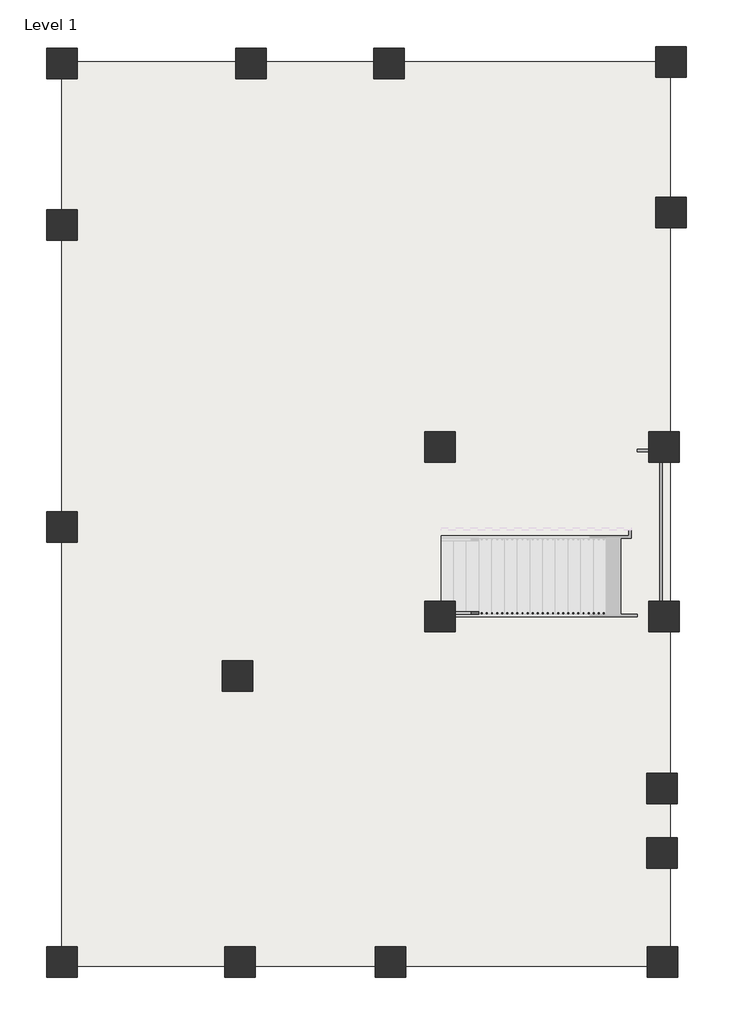
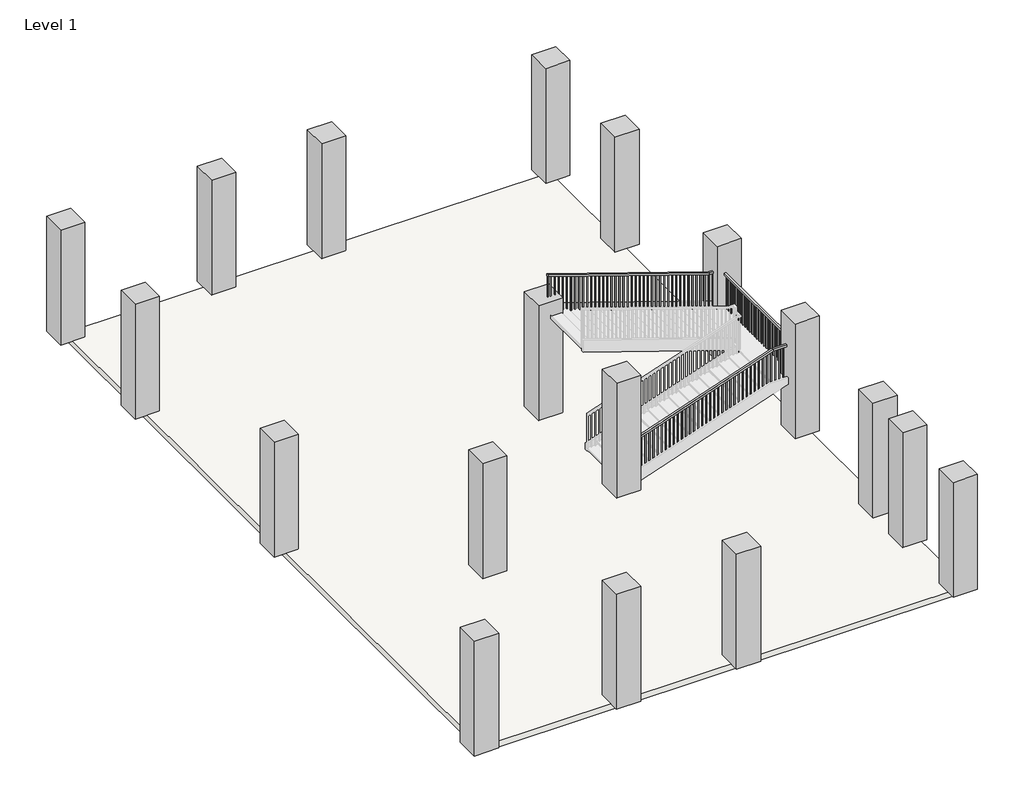
# One storey, part 1 of 2: 18 columns, 1 railing, 1 slab.
"""IFC4 building model written with IfcOpenShell, lengths in millimetres."""

from ifc_helpers import new_model, si_unit, frame, origin, origin_with_axes, place, context, project, spatial, polyline, outline, extrude, faceted_brep, element, save

model = new_model("IFC4")

# Units and contexts
model_context = context("Model", 3, world=origin())
ifc_project = project(units=[si_unit("LENGTHUNIT", "METRE", prefix="MILLI")], contexts=[model_context])

# Site, building, storey
site = spatial("IfcSite", under=ifc_project)
building = spatial("IfcBuilding", under=site)
storey = spatial("IfcBuildingStorey", under=building, Name="Level 1", Elevation=0.0)

# Columns
placement = place(None, origin())
element("IfcColumn", 1, ObjectType="Rectangular Column : 9\"x12\"/12\"x12\"", at=placement, inside=storey, context=model_context, shape_type="SweptSolid", body=[
    extrude(outline(polyline([(-5829.2560205, 9252.6670151), (-5829.2560205, 8643.0670151), (-6438.8560205, 8643.0670151), (-6438.8560205, 9252.6670151), (-5829.2560205, 9252.6670151)])), origin_with_axes(), (0.0, 0.0, 1.0), 3048.0),
])
element("IfcColumn", 2, ObjectType="Rectangular Column : 9\"x12\"/12\"x12\"", at=placement, inside=storey, context=model_context, shape_type="SweptSolid", body=[
    extrude(outline(polyline([(6350.6915654, 9284.2113669), (6350.6915654, 8674.6113669), (5741.0915654, 8674.6113669), (5741.0915654, 9284.2113669), (6350.6915654, 9284.2113669)])), origin_with_axes(), (0.0, 0.0, 1.0), 3048.0),
])
element("IfcColumn", 3, ObjectType="Rectangular Column : 9\"x12\"/12\"x12\"", at=placement, inside=storey, context=model_context, shape_type="SweptSolid", body=[
    extrude(outline(polyline([(-2044.6166288, 9252.6670151), (-2044.6166288, 8643.0670151), (-2654.2166288, 8643.0670151), (-2654.2166288, 9252.6670151), (-2044.6166288, 9252.6670151)])), origin_with_axes(), (0.0, 0.0, 1.0), 3048.0),
])
element("IfcColumn", 4, ObjectType="Rectangular Column : 9\"x12\"/12\"x12\"", at=placement, inside=storey, context=model_context, shape_type="SweptSolid", body=[
    extrude(outline(polyline([(713.9012016, 9252.6670151), (713.9012016, 8643.0670151), (104.3012016, 8643.0670151), (104.3012016, 9252.6670151), (713.9012016, 9252.6670151)])), origin_with_axes(), (0.0, 0.0, 1.0), 3048.0),
])
element("IfcColumn", 5, ObjectType="Rectangular Column : 9\"x12\"/12\"x12\"", at=placement, inside=storey, context=model_context, shape_type="SweptSolid", body=[
    extrude(outline(polyline([(-5829.2560205, 6018.6061457), (-5829.2560205, 5409.0061457), (-6438.8560205, 5409.0061457), (-6438.8560205, 6018.6061457), (-5829.2560205, 6018.6061457)])), origin_with_axes(), (0.0, 0.0, 1.0), 3048.0),
])
element("IfcColumn", 6, ObjectType="Rectangular Column : 9\"x12\"/12\"x12\"", at=placement, inside=storey, context=model_context, shape_type="SweptSolid", body=[
    extrude(outline(polyline([(-5829.1978401, -18.1127424), (-5829.1978401, -627.7127424), (-6438.7978401, -627.7127424), (-6438.7978401, -18.1127424), (-5829.1978401, -18.1127424)])), origin_with_axes(), (0.0, 0.0, 1.0), 3048.0),
])
element("IfcColumn", 7, ObjectType="Rectangular Column : 9\"x12\"/12\"x12\"", at=placement, inside=storey, context=model_context, shape_type="SweptSolid", body=[
    extrude(outline(polyline([(-5826.9839448, -8713.9734342), (-5826.9839448, -9323.5734342), (-6436.5839448, -9323.5734342), (-6436.5839448, -8713.9734342), (-5826.9839448, -8713.9734342)])), origin_with_axes(), (0.0, 0.0, 1.0), 3048.0),
])
element("IfcColumn", 8, ObjectType="Rectangular Column : 9\"x12\"/12\"x12\"", at=placement, inside=storey, context=model_context, shape_type="SweptSolid", body=[
    extrude(outline(polyline([(-2270.3220989, -8713.9734342), (-2270.3220989, -9323.5734342), (-2879.9220989, -9323.5734342), (-2879.9220989, -8713.9734342), (-2270.3220989, -8713.9734342)])), origin_with_axes(), (0.0, 0.0, 1.0), 3048.0),
])
element("IfcColumn", 9, ObjectType="Rectangular Column : 9\"x12\"/12\"x12\"", at=placement, inside=storey, context=model_context, shape_type="SweptSolid", body=[
    extrude(outline(polyline([(745.5939638, -8713.9734342), (745.5939638, -9323.5734342), (135.9939638, -9323.5734342), (135.9939638, -8713.9734342), (745.5939638, -8713.9734342)])), origin_with_axes(), (0.0, 0.0, 1.0), 3048.0),
])
element("IfcColumn", 10, ObjectType="Rectangular Column : 9\"x12\"/12\"x12\"", at=placement, inside=storey, context=model_context, shape_type="SweptSolid", body=[
    extrude(outline(polyline([(6178.8473287, -8713.9734342), (6178.8473287, -9323.5734342), (5569.2473287, -9323.5734342), (5569.2473287, -8713.9734342), (6178.8473287, -8713.9734342)])), origin_with_axes(), (0.0, 0.0, 1.0), 3048.0),
])
element("IfcColumn", 11, ObjectType="Rectangular Column : 9\"x12\"/12\"x12\"", at=placement, inside=storey, context=model_context, shape_type="SweptSolid", body=[
    extrude(outline(polyline([(6172.2396412, -6530.895318), (6172.2396412, -7140.495318), (5562.6396412, -7140.495318), (5562.6396412, -6530.895318), (6172.2396412, -6530.895318)])), origin_with_axes(), (0.0, 0.0, 1.0), 3048.0),
])
element("IfcColumn", 12, ObjectType="Rectangular Column : 9\"x12\"/12\"x12\"", at=placement, inside=storey, context=model_context, shape_type="SweptSolid", body=[
    extrude(outline(polyline([(6172.2396412, -5240.916233), (6172.2396412, -5850.516233), (5562.6396412, -5850.516233), (5562.6396412, -5240.916233), (6172.2396412, -5240.916233)])), origin_with_axes(), (0.0, 0.0, 1.0), 3048.0),
])
element("IfcColumn", 13, ObjectType="Rectangular Column : 9\"x12\"/12\"x12\"", at=placement, inside=storey, context=model_context, shape_type="SweptSolid", body=[
    extrude(outline(polyline([(6208.2949572, -1801.6977001), (6208.2949572, -2411.2977001), (5598.6949572, -2411.2977001), (5598.6949572, -1801.6977001), (6208.2949572, -1801.6977001)])), origin_with_axes(), (0.0, 0.0, 1.0), 3048.0),
])
element("IfcColumn", 14, ObjectType="Rectangular Column : 9\"x12\"/12\"x12\"", at=placement, inside=storey, context=model_context, shape_type="SweptSolid", body=[
    extrude(outline(polyline([(6208.2949572, 1586.0589984), (6208.2949572, 976.4589984), (5598.6949572, 976.4589984), (5598.6949572, 1586.0589984), (6208.2949572, 1586.0589984)])), origin_with_axes(), (0.0, 0.0, 1.0), 3048.0),
])
element("IfcColumn", 15, ObjectType="Rectangular Column : 9\"x12\"/12\"x12\"", at=placement, inside=storey, context=model_context, shape_type="SweptSolid", body=[
    extrude(outline(polyline([(6350.6915654, 6275.5882388), (6350.6915654, 5665.9882388), (5741.0915654, 5665.9882388), (5741.0915654, 6275.5882388), (6350.6915654, 6275.5882388)])), origin_with_axes(), (0.0, 0.0, 1.0), 3048.0),
])
element("IfcColumn", 16, ObjectType="Rectangular Column : 9\"x12\"/12\"x12\"", at=placement, inside=storey, context=model_context, shape_type="SweptSolid", body=[
    extrude(outline(polyline([(1728.7932247, 1586.0589984), (1728.7932247, 976.4589984), (1119.1932247, 976.4589984), (1119.1932247, 1586.0589984), (1728.7932247, 1586.0589984)])), origin_with_axes(), (0.0, 0.0, 1.0), 3048.0),
])
element("IfcColumn", 17, ObjectType="Rectangular Column : 9\"x12\"/12\"x12\"", at=placement, inside=storey, context=model_context, shape_type="SweptSolid", body=[
    extrude(outline(polyline([(1728.7932247, -1801.6977001), (1728.7932247, -2411.2977001), (1119.1932247, -2411.2977001), (1119.1932247, -1801.6977001), (1728.7932247, -1801.6977001)])), origin_with_axes(), (0.0, 0.0, 1.0), 3048.0),
])
element("IfcColumn", 18, ObjectType="Rectangular Column : 9\"x12\"/12\"x12\"", at=placement, inside=storey, context=model_context, shape_type="SweptSolid", body=[
    extrude(outline(polyline([(-2316.8197661, -2995.5861861), (-2316.8197661, -3605.1861861), (-2926.4197661, -3605.1861861), (-2926.4197661, -2995.5861861), (-2316.8197661, -2995.5861861)])), origin_with_axes(), (0.0, 0.0, 1.0), 3048.0),
])

# Railing
element("IfcRailing", 19, ObjectType="Handrail - Rectangular", at=placement, inside=storey, context=model_context, shape_type="SolidModel", body=[
    faceted_brep([(1449.3932247, -2014.4659014, 1000.125), (1449.3932247, -2014.4659014, 946.4913852), (1449.3932247, -2065.2659014, 946.4913852), (1449.3932247, -2065.2659014, 1000.125), (5246.6669505, -2014.4659014, 2286.0), (5255.0348019, -2014.4659014, 2235.2), (5255.0348019, -2065.2659014, 2235.2), (5246.6669505, -2065.2659014, 2286.0), (5771.4548051, -2014.4659014, 2286.0), (5771.4548051, -2014.4659014, 2235.2), (5822.2548051, -2065.2659014, 2235.2), (5822.2548051, -2065.2659014, 2286.0), (5771.4548051, 1135.1340986, 2286.0), (5771.4548051, 1135.1340986, 2235.2), (5822.2548051, 1185.9340986, 2235.2), (5822.2548051, 1185.9340986, 2286.0), (5499.8185322, 1135.1340986, 2286.0), (5491.4506807, 1135.1340986, 2235.2), (5491.4506807, 1185.9340986, 2235.2), (5499.8185322, 1185.9340986, 2286.0), (1449.3932247, 1135.1340986, 3657.6), (1449.3932247, 1185.9340986, 3657.6), (1449.3932247, 1185.9340986, 3603.9663852), (1449.3932247, 1135.1340986, 3603.9663852)], [[[0, 1, 2, 3]], [[1, 0, 4, 5]], [[2, 1, 5, 6]], [[3, 2, 6, 7]], [[0, 3, 7, 4]], [[5, 4, 8, 9]], [[6, 5, 9, 10]], [[7, 6, 10, 11]], [[4, 7, 11, 8]], [[9, 8, 12, 13]], [[10, 9, 13, 14]], [[11, 10, 14, 15]], [[8, 11, 15, 12]], [[13, 12, 16, 17]], [[14, 13, 17, 18]], [[15, 14, 18, 19]], [[12, 15, 19, 16]], [[20, 21, 22, 23]], [[17, 16, 20, 23]], [[18, 17, 23, 22]], [[19, 18, 22, 21]], [[16, 19, 21, 20]]]),
    extrude(outline(polyline([(3573.5618562, 1539.1798051), (3580.0127788, 1520.1298051), (2657.475, 1520.1298051), (2657.475, 1539.1798051), (3573.5618562, 1539.1798051)])), frame((0.0, 1151.0090986, 0.0), z_axis=(0.0, 1.0, 0.0), x_axis=(0.0, 0.0, 1.0)), (0.0, 0.0, 1.0), 19.05),
    extrude(outline(polyline([(3539.1569359, 1640.7798051), (3545.6078585, 1621.7298051), (2657.475, 1621.7298051), (2657.475, 1640.7798051), (3539.1569359, 1640.7798051)])), frame((0.0, 1151.0090986, 0.0), z_axis=(0.0, 1.0, 0.0), x_axis=(0.0, 0.0, 1.0)), (0.0, 0.0, 1.0), 19.05),
    extrude(outline(polyline([(3504.7520156, 1742.3798051), (3511.2029381, 1723.3298051), (2571.75, 1723.3298051), (2571.75, 1742.3798051), (3504.7520156, 1742.3798051)])), frame((0.0, 1151.0090986, 0.0), z_axis=(0.0, 1.0, 0.0), x_axis=(0.0, 0.0, 1.0)), (0.0, 0.0, 1.0), 19.05),
    extrude(outline(polyline([(3470.3470953, 1843.9798051), (3476.7980178, 1824.9298051), (2571.75, 1824.9298051), (2571.75, 1843.9798051), (3470.3470953, 1843.9798051)])), frame((0.0, 1151.0090986, 0.0), z_axis=(0.0, 1.0, 0.0), x_axis=(0.0, 0.0, 1.0)), (0.0, 0.0, 1.0), 19.05),
    extrude(outline(polyline([(3435.9421749, 1945.5798051), (3442.3930975, 1926.5298051), (2571.75, 1926.5298051), (2571.75, 1945.5798051), (3435.9421749, 1945.5798051)])), frame((0.0, 1151.0090986, 0.0), z_axis=(0.0, 1.0, 0.0), x_axis=(0.0, 0.0, 1.0)), (0.0, 0.0, 1.0), 19.05),
    extrude(outline(polyline([(3401.5372546, 2047.1798051), (3407.9881772, 2028.1298051), (2486.025, 2028.1298051), (2486.025, 2047.1798051), (3401.5372546, 2047.1798051)])), frame((0.0, 1151.0090986, 0.0), z_axis=(0.0, 1.0, 0.0), x_axis=(0.0, 0.0, 1.0)), (0.0, 0.0, 1.0), 19.05),
    extrude(outline(polyline([(3367.1323343, 2148.7798051), (3373.5832568, 2129.7298051), (2486.025, 2129.7298051), (2486.025, 2148.7798051), (3367.1323343, 2148.7798051)])), frame((0.0, 1151.0090986, 0.0), z_axis=(0.0, 1.0, 0.0), x_axis=(0.0, 0.0, 1.0)), (0.0, 0.0, 1.0), 19.05),
    extrude(outline(polyline([(3332.7274139, 2250.3798051), (3339.1783365, 2231.3298051), (2400.3, 2231.3298051), (2400.3, 2250.3798051), (3332.7274139, 2250.3798051)])), frame((0.0, 1151.0090986, 0.0), z_axis=(0.0, 1.0, 0.0), x_axis=(0.0, 0.0, 1.0)), (0.0, 0.0, 1.0), 19.05),
    extrude(outline(polyline([(3298.3224936, 2351.9798051), (3304.7734162, 2332.9298051), (2400.3, 2332.9298051), (2400.3, 2351.9798051), (3298.3224936, 2351.9798051)])), frame((0.0, 1151.0090986, 0.0), z_axis=(0.0, 1.0, 0.0), x_axis=(0.0, 0.0, 1.0)), (0.0, 0.0, 1.0), 19.05),
    extrude(outline(polyline([(3263.9175733, 2453.5798051), (3270.3684958, 2434.5298051), (2400.3, 2434.5298051), (2400.3, 2453.5798051), (3263.9175733, 2453.5798051)])), frame((0.0, 1151.0090986, 0.0), z_axis=(0.0, 1.0, 0.0), x_axis=(0.0, 0.0, 1.0)), (0.0, 0.0, 1.0), 19.05),
    extrude(outline(polyline([(3229.512653, 2555.1798051), (3235.9635755, 2536.1298051), (2314.575, 2536.1298051), (2314.575, 2555.1798051), (3229.512653, 2555.1798051)])), frame((0.0, 1151.0090986, 0.0), z_axis=(0.0, 1.0, 0.0), x_axis=(0.0, 0.0, 1.0)), (0.0, 0.0, 1.0), 19.05),
    extrude(outline(polyline([(3195.1077326, 2656.7798051), (3201.5586552, 2637.7298051), (2314.575, 2637.7298051), (2314.575, 2656.7798051), (3195.1077326, 2656.7798051)])), frame((0.0, 1151.0090986, 0.0), z_axis=(0.0, 1.0, 0.0), x_axis=(0.0, 0.0, 1.0)), (0.0, 0.0, 1.0), 19.05),
    extrude(outline(polyline([(3160.7028123, 2758.3798051), (3167.1537349, 2739.3298051), (2228.85, 2739.3298051), (2228.85, 2758.3798051), (3160.7028123, 2758.3798051)])), frame((0.0, 1151.0090986, 0.0), z_axis=(0.0, 1.0, 0.0), x_axis=(0.0, 0.0, 1.0)), (0.0, 0.0, 1.0), 19.05),
    extrude(outline(polyline([(3126.297892, 2859.9798051), (3132.7488145, 2840.9298051), (2228.85, 2840.9298051), (2228.85, 2859.9798051), (3126.297892, 2859.9798051)])), frame((0.0, 1151.0090986, 0.0), z_axis=(0.0, 1.0, 0.0), x_axis=(0.0, 0.0, 1.0)), (0.0, 0.0, 1.0), 19.05),
    extrude(outline(polyline([(3091.8929716, 2961.5798051), (3098.3438942, 2942.5298051), (2228.85, 2942.5298051), (2228.85, 2961.5798051), (3091.8929716, 2961.5798051)])), frame((0.0, 1151.0090986, 0.0), z_axis=(0.0, 1.0, 0.0), x_axis=(0.0, 0.0, 1.0)), (0.0, 0.0, 1.0), 19.05),
    extrude(outline(polyline([(3057.4880513, 3063.1798051), (3063.9389739, 3044.1298051), (2143.125, 3044.1298051), (2143.125, 3063.1798051), (3057.4880513, 3063.1798051)])), frame((0.0, 1151.0090986, 0.0), z_axis=(0.0, 1.0, 0.0), x_axis=(0.0, 0.0, 1.0)), (0.0, 0.0, 1.0), 19.05),
    extrude(outline(polyline([(3023.083131, 3164.7798051), (3029.5340535, 3145.7298051), (2143.125, 3145.7298051), (2143.125, 3164.7798051), (3023.083131, 3164.7798051)])), frame((0.0, 1151.0090986, 0.0), z_axis=(0.0, 1.0, 0.0), x_axis=(0.0, 0.0, 1.0)), (0.0, 0.0, 1.0), 19.05),
    extrude(outline(polyline([(2988.6782106, 3266.3798051), (2995.1291332, 3247.3298051), (2057.4, 3247.3298051), (2057.4, 3266.3798051), (2988.6782106, 3266.3798051)])), frame((0.0, 1151.0090986, 0.0), z_axis=(0.0, 1.0, 0.0), x_axis=(0.0, 0.0, 1.0)), (0.0, 0.0, 1.0), 19.05),
    extrude(outline(polyline([(2954.2732903, 3367.9798051), (2960.7242129, 3348.9298051), (2057.4, 3348.9298051), (2057.4, 3367.9798051), (2954.2732903, 3367.9798051)])), frame((0.0, 1151.0090986, 0.0), z_axis=(0.0, 1.0, 0.0), x_axis=(0.0, 0.0, 1.0)), (0.0, 0.0, 1.0), 19.05),
    extrude(outline(polyline([(2919.86837, 3469.5798051), (2926.3192926, 3450.5298051), (2057.4, 3450.5298051), (2057.4, 3469.5798051), (2919.86837, 3469.5798051)])), frame((0.0, 1151.0090986, 0.0), z_axis=(0.0, 1.0, 0.0), x_axis=(0.0, 0.0, 1.0)), (0.0, 0.0, 1.0), 19.05),
    extrude(outline(polyline([(2885.4634497, 3571.1798051), (2891.9143722, 3552.1298051), (1971.675, 3552.1298051), (1971.675, 3571.1798051), (2885.4634497, 3571.1798051)])), frame((0.0, 1151.0090986, 0.0), z_axis=(0.0, 1.0, 0.0), x_axis=(0.0, 0.0, 1.0)), (0.0, 0.0, 1.0), 19.05),
    extrude(outline(polyline([(2851.0585293, 3672.7798051), (2857.5094519, 3653.7298051), (1971.675, 3653.7298051), (1971.675, 3672.7798051), (2851.0585293, 3672.7798051)])), frame((0.0, 1151.0090986, 0.0), z_axis=(0.0, 1.0, 0.0), x_axis=(0.0, 0.0, 1.0)), (0.0, 0.0, 1.0), 19.05),
    extrude(outline(polyline([(2816.653609, 3774.3798051), (2823.1045316, 3755.3298051), (1885.95, 3755.3298051), (1885.95, 3774.3798051), (2816.653609, 3774.3798051)])), frame((0.0, 1151.0090986, 0.0), z_axis=(0.0, 1.0, 0.0), x_axis=(0.0, 0.0, 1.0)), (0.0, 0.0, 1.0), 19.05),
    extrude(outline(polyline([(2782.2486887, 3875.9798051), (2788.6996112, 3856.9298051), (1885.95, 3856.9298051), (1885.95, 3875.9798051), (2782.2486887, 3875.9798051)])), frame((0.0, 1151.0090986, 0.0), z_axis=(0.0, 1.0, 0.0), x_axis=(0.0, 0.0, 1.0)), (0.0, 0.0, 1.0), 19.05),
    extrude(outline(polyline([(2747.8437683, 3977.5798051), (2754.2946909, 3958.5298051), (1885.95, 3958.5298051), (1885.95, 3977.5798051), (2747.8437683, 3977.5798051)])), frame((0.0, 1151.0090986, 0.0), z_axis=(0.0, 1.0, 0.0), x_axis=(0.0, 0.0, 1.0)), (0.0, 0.0, 1.0), 19.05),
    extrude(outline(polyline([(2713.438848, 4079.1798051), (2719.8897706, 4060.1298051), (1800.225, 4060.1298051), (1800.225, 4079.1798051), (2713.438848, 4079.1798051)])), frame((0.0, 1151.0090986, 0.0), z_axis=(0.0, 1.0, 0.0), x_axis=(0.0, 0.0, 1.0)), (0.0, 0.0, 1.0), 19.05),
    extrude(outline(polyline([(2679.0339277, 4180.7798051), (2685.4848503, 4161.7298051), (1800.225, 4161.7298051), (1800.225, 4180.7798051), (2679.0339277, 4180.7798051)])), frame((0.0, 1151.0090986, 0.0), z_axis=(0.0, 1.0, 0.0), x_axis=(0.0, 0.0, 1.0)), (0.0, 0.0, 1.0), 19.05),
    extrude(outline(polyline([(2644.6290074, 4282.3798051), (2651.0799299, 4263.3298051), (1714.5, 4263.3298051), (1714.5, 4282.3798051), (2644.6290074, 4282.3798051)])), frame((0.0, 1151.0090986, 0.0), z_axis=(0.0, 1.0, 0.0), x_axis=(0.0, 0.0, 1.0)), (0.0, 0.0, 1.0), 19.05),
    extrude(outline(polyline([(2610.224087, 4383.9798051), (2616.6750096, 4364.9298051), (1714.5, 4364.9298051), (1714.5, 4383.9798051), (2610.224087, 4383.9798051)])), frame((0.0, 1151.0090986, 0.0), z_axis=(0.0, 1.0, 0.0), x_axis=(0.0, 0.0, 1.0)), (0.0, 0.0, 1.0), 19.05),
    extrude(outline(polyline([(2575.8191667, 4485.5798051), (2582.2700893, 4466.5298051), (1714.5, 4466.5298051), (1714.5, 4485.5798051), (2575.8191667, 4485.5798051)])), frame((0.0, 1151.0090986, 0.0), z_axis=(0.0, 1.0, 0.0), x_axis=(0.0, 0.0, 1.0)), (0.0, 0.0, 1.0), 19.05),
    extrude(outline(polyline([(2541.4142464, 4587.1798051), (2547.8651689, 4568.1298051), (1628.775, 4568.1298051), (1628.775, 4587.1798051), (2541.4142464, 4587.1798051)])), frame((0.0, 1151.0090986, 0.0), z_axis=(0.0, 1.0, 0.0), x_axis=(0.0, 0.0, 1.0)), (0.0, 0.0, 1.0), 19.05),
    extrude(outline(polyline([(2507.009326, 4688.7798051), (2513.4602486, 4669.7298051), (1628.775, 4669.7298051), (1628.775, 4688.7798051), (2507.009326, 4688.7798051)])), frame((0.0, 1151.0090986, 0.0), z_axis=(0.0, 1.0, 0.0), x_axis=(0.0, 0.0, 1.0)), (0.0, 0.0, 1.0), 19.05),
    extrude(outline(polyline([(2472.6044057, 4790.3798051), (2479.0553283, 4771.3298051), (1543.05, 4771.3298051), (1543.05, 4790.3798051), (2472.6044057, 4790.3798051)])), frame((0.0, 1151.0090986, 0.0), z_axis=(0.0, 1.0, 0.0), x_axis=(0.0, 0.0, 1.0)), (0.0, 0.0, 1.0), 19.05),
    extrude(outline(polyline([(2438.1994854, 4891.9798051), (2444.6504079, 4872.9298051), (1543.05, 4872.9298051), (1543.05, 4891.9798051), (2438.1994854, 4891.9798051)])), frame((0.0, 1151.0090986, 0.0), z_axis=(0.0, 1.0, 0.0), x_axis=(0.0, 0.0, 1.0)), (0.0, 0.0, 1.0), 19.05),
    extrude(outline(polyline([(2403.8163852, 4993.5798051), (2410.2673078, 4974.5298051), (1543.05, 4974.5298051), (1543.05, 4993.5798051), (2403.8163852, 4993.5798051)])), frame((0.0, 1151.0090986, 0.0), z_axis=(0.0, 1.0, 0.0), x_axis=(0.0, 0.0, 1.0)), (0.0, 0.0, 1.0), 19.05),
    extrude(outline(polyline([(2369.3896447, 5095.1798051), (2375.8405673, 5076.1298051), (1457.325, 5076.1298051), (1457.325, 5095.1798051), (2369.3896447, 5095.1798051)])), frame((0.0, 1151.0090986, 0.0), z_axis=(0.0, 1.0, 0.0), x_axis=(0.0, 0.0, 1.0)), (0.0, 0.0, 1.0), 19.05),
    extrude(outline(polyline([(2334.9847244, 5196.7798051), (2341.435647, 5177.7298051), (1457.325, 5177.7298051), (1457.325, 5196.7798051), (2334.9847244, 5196.7798051)])), frame((0.0, 1151.0090986, 0.0), z_axis=(0.0, 1.0, 0.0), x_axis=(0.0, 0.0, 1.0)), (0.0, 0.0, 1.0), 19.05),
    extrude(outline(polyline([(2300.5798041, 5298.3798051), (2307.0307266, 5279.3298051), (1371.6, 5279.3298051), (1371.6, 5298.3798051), (2300.5798041, 5298.3798051)])), frame((0.0, 1151.0090986, 0.0), z_axis=(0.0, 1.0, 0.0), x_axis=(0.0, 0.0, 1.0)), (0.0, 0.0, 1.0), 19.05),
    extrude(outline(polyline([(2266.1748837, 5399.9798051), (2272.6258063, 5380.9298051), (1371.6, 5380.9298051), (1371.6, 5399.9798051), (2266.1748837, 5399.9798051)])), frame((0.0, 1151.0090986, 0.0), z_axis=(0.0, 1.0, 0.0), x_axis=(0.0, 0.0, 1.0)), (0.0, 0.0, 1.0), 19.05),
    extrude(outline(polyline([(2231.7699634, 5501.5798051), (2238.220886, 5482.5298051), (1371.6, 5482.5298051), (1371.6, 5501.5798051), (2231.7699634, 5501.5798051)])), frame((0.0, 1151.0090986, 0.0), z_axis=(0.0, 1.0, 0.0), x_axis=(0.0, 0.0, 1.0)), (0.0, 0.0, 1.0), 19.05),
    extrude(outline(polyline([(5603.1798051, 1170.0590986), (5603.1798051, 1151.0090986), (5584.1298051, 1151.0090986), (5584.1298051, 1170.0590986), (5603.1798051, 1170.0590986)])), frame((0.0, 0.0, 1371.6), z_axis=(0.0, 0.0, 1.0), x_axis=(1.0, 0.0, 0.0)), (0.0, 0.0, 1.0), 863.6),
    extrude(outline(polyline([(5704.7798051, 1170.0590986), (5704.7798051, 1151.0090986), (5685.7298051, 1151.0090986), (5685.7298051, 1170.0590986), (5704.7798051, 1170.0590986)])), frame((0.0, 0.0, 1371.6), z_axis=(0.0, 0.0, 1.0), x_axis=(1.0, 0.0, 0.0)), (0.0, 0.0, 1.0), 863.6),
    extrude(outline(polyline([(5806.3798051, 1100.2090986), (5787.3298051, 1100.2090986), (5787.3298051, 1119.2590986), (5806.3798051, 1119.2590986), (5806.3798051, 1100.2090986)])), frame((0.0, 0.0, 1371.6), z_axis=(0.0, 0.0, 1.0), x_axis=(1.0, 0.0, 0.0)), (0.0, 0.0, 1.0), 863.6),
    extrude(outline(polyline([(5806.3798051, 998.6090986), (5787.3298051, 998.6090986), (5787.3298051, 1017.6590986), (5806.3798051, 1017.6590986), (5806.3798051, 998.6090986)])), frame((0.0, 0.0, 1371.6), z_axis=(0.0, 0.0, 1.0), x_axis=(1.0, 0.0, 0.0)), (0.0, 0.0, 1.0), 863.6),
    extrude(outline(polyline([(5806.3798051, 897.0090986), (5787.3298051, 897.0090986), (5787.3298051, 916.0590986), (5806.3798051, 916.0590986), (5806.3798051, 897.0090986)])), frame((0.0, 0.0, 1371.6), z_axis=(0.0, 0.0, 1.0), x_axis=(1.0, 0.0, 0.0)), (0.0, 0.0, 1.0), 863.6),
    extrude(outline(polyline([(5806.3798051, 795.4090986), (5787.3298051, 795.4090986), (5787.3298051, 814.4590986), (5806.3798051, 814.4590986), (5806.3798051, 795.4090986)])), frame((0.0, 0.0, 1371.6), z_axis=(0.0, 0.0, 1.0), x_axis=(1.0, 0.0, 0.0)), (0.0, 0.0, 1.0), 863.6),
    extrude(outline(polyline([(5806.3798051, 693.8090986), (5787.3298051, 693.8090986), (5787.3298051, 712.8590986), (5806.3798051, 712.8590986), (5806.3798051, 693.8090986)])), frame((0.0, 0.0, 1371.6), z_axis=(0.0, 0.0, 1.0), x_axis=(1.0, 0.0, 0.0)), (0.0, 0.0, 1.0), 863.6),
    extrude(outline(polyline([(5806.3798051, 592.2090986), (5787.3298051, 592.2090986), (5787.3298051, 611.2590986), (5806.3798051, 611.2590986), (5806.3798051, 592.2090986)])), frame((0.0, 0.0, 1371.6), z_axis=(0.0, 0.0, 1.0), x_axis=(1.0, 0.0, 0.0)), (0.0, 0.0, 1.0), 863.6),
    extrude(outline(polyline([(5806.3798051, 490.6090986), (5787.3298051, 490.6090986), (5787.3298051, 509.6590986), (5806.3798051, 509.6590986), (5806.3798051, 490.6090986)])), frame((0.0, 0.0, 1371.6), z_axis=(0.0, 0.0, 1.0), x_axis=(1.0, 0.0, 0.0)), (0.0, 0.0, 1.0), 863.6),
    extrude(outline(polyline([(5806.3798051, 389.0090986), (5787.3298051, 389.0090986), (5787.3298051, 408.0590986), (5806.3798051, 408.0590986), (5806.3798051, 389.0090986)])), frame((0.0, 0.0, 1371.6), z_axis=(0.0, 0.0, 1.0), x_axis=(1.0, 0.0, 0.0)), (0.0, 0.0, 1.0), 863.6),
    extrude(outline(polyline([(5806.3798051, 287.4090986), (5787.3298051, 287.4090986), (5787.3298051, 306.4590986), (5806.3798051, 306.4590986), (5806.3798051, 287.4090986)])), frame((0.0, 0.0, 1371.6), z_axis=(0.0, 0.0, 1.0), x_axis=(1.0, 0.0, 0.0)), (0.0, 0.0, 1.0), 863.6),
    extrude(outline(polyline([(5806.3798051, 185.8090986), (5787.3298051, 185.8090986), (5787.3298051, 204.8590986), (5806.3798051, 204.8590986), (5806.3798051, 185.8090986)])), frame((0.0, 0.0, 1371.6), z_axis=(0.0, 0.0, 1.0), x_axis=(1.0, 0.0, 0.0)), (0.0, 0.0, 1.0), 863.6),
    extrude(outline(polyline([(5806.3798051, 84.2090986), (5787.3298051, 84.2090986), (5787.3298051, 103.2590986), (5806.3798051, 103.2590986), (5806.3798051, 84.2090986)])), frame((0.0, 0.0, 1371.6), z_axis=(0.0, 0.0, 1.0), x_axis=(1.0, 0.0, 0.0)), (0.0, 0.0, 1.0), 863.6),
    extrude(outline(polyline([(5806.3798051, -17.3909014), (5787.3298051, -17.3909014), (5787.3298051, 1.6590986), (5806.3798051, 1.6590986), (5806.3798051, -17.3909014)])), frame((0.0, 0.0, 1371.6), z_axis=(0.0, 0.0, 1.0), x_axis=(1.0, 0.0, 0.0)), (0.0, 0.0, 1.0), 863.6),
    extrude(outline(polyline([(5806.3798051, -118.9909014), (5787.3298051, -118.9909014), (5787.3298051, -99.9409014), (5806.3798051, -99.9409014), (5806.3798051, -118.9909014)])), frame((0.0, 0.0, 1371.6), z_axis=(0.0, 0.0, 1.0), x_axis=(1.0, 0.0, 0.0)), (0.0, 0.0, 1.0), 863.6),
    extrude(outline(polyline([(5806.3798051, -220.5909014), (5787.3298051, -220.5909014), (5787.3298051, -201.5409014), (5806.3798051, -201.5409014), (5806.3798051, -220.5909014)])), frame((0.0, 0.0, 1371.6), z_axis=(0.0, 0.0, 1.0), x_axis=(1.0, 0.0, 0.0)), (0.0, 0.0, 1.0), 863.6),
    extrude(outline(polyline([(5806.3798051, -322.1909014), (5787.3298051, -322.1909014), (5787.3298051, -303.1409014), (5806.3798051, -303.1409014), (5806.3798051, -322.1909014)])), frame((0.0, 0.0, 1371.6), z_axis=(0.0, 0.0, 1.0), x_axis=(1.0, 0.0, 0.0)), (0.0, 0.0, 1.0), 863.6),
    extrude(outline(polyline([(5806.3798051, -423.7909014), (5787.3298051, -423.7909014), (5787.3298051, -404.7409014), (5806.3798051, -404.7409014), (5806.3798051, -423.7909014)])), frame((0.0, 0.0, 1371.6), z_axis=(0.0, 0.0, 1.0), x_axis=(1.0, 0.0, 0.0)), (0.0, 0.0, 1.0), 863.6),
    extrude(outline(polyline([(5806.3798051, -525.3909014), (5787.3298051, -525.3909014), (5787.3298051, -506.3409014), (5806.3798051, -506.3409014), (5806.3798051, -525.3909014)])), frame((0.0, 0.0, 1371.6), z_axis=(0.0, 0.0, 1.0), x_axis=(1.0, 0.0, 0.0)), (0.0, 0.0, 1.0), 863.6),
    extrude(outline(polyline([(5806.3798051, -626.9909014), (5787.3298051, -626.9909014), (5787.3298051, -607.9409014), (5806.3798051, -607.9409014), (5806.3798051, -626.9909014)])), frame((0.0, 0.0, 1371.6), z_axis=(0.0, 0.0, 1.0), x_axis=(1.0, 0.0, 0.0)), (0.0, 0.0, 1.0), 863.6),
    extrude(outline(polyline([(5806.3798051, -728.5909014), (5787.3298051, -728.5909014), (5787.3298051, -709.5409014), (5806.3798051, -709.5409014), (5806.3798051, -728.5909014)])), frame((0.0, 0.0, 1371.6), z_axis=(0.0, 0.0, 1.0), x_axis=(1.0, 0.0, 0.0)), (0.0, 0.0, 1.0), 863.6),
    extrude(outline(polyline([(5806.3798051, -830.1909014), (5787.3298051, -830.1909014), (5787.3298051, -811.1409014), (5806.3798051, -811.1409014), (5806.3798051, -830.1909014)])), frame((0.0, 0.0, 1371.6), z_axis=(0.0, 0.0, 1.0), x_axis=(1.0, 0.0, 0.0)), (0.0, 0.0, 1.0), 863.6),
    extrude(outline(polyline([(5806.3798051, -931.7909014), (5787.3298051, -931.7909014), (5787.3298051, -912.7409014), (5806.3798051, -912.7409014), (5806.3798051, -931.7909014)])), frame((0.0, 0.0, 1371.6), z_axis=(0.0, 0.0, 1.0), x_axis=(1.0, 0.0, 0.0)), (0.0, 0.0, 1.0), 863.6),
    extrude(outline(polyline([(5806.3798051, -1033.3909014), (5787.3298051, -1033.3909014), (5787.3298051, -1014.3409014), (5806.3798051, -1014.3409014), (5806.3798051, -1033.3909014)])), frame((0.0, 0.0, 1371.6), z_axis=(0.0, 0.0, 1.0), x_axis=(1.0, 0.0, 0.0)), (0.0, 0.0, 1.0), 863.6),
    extrude(outline(polyline([(5806.3798051, -1134.9909014), (5787.3298051, -1134.9909014), (5787.3298051, -1115.9409014), (5806.3798051, -1115.9409014), (5806.3798051, -1134.9909014)])), frame((0.0, 0.0, 1371.6), z_axis=(0.0, 0.0, 1.0), x_axis=(1.0, 0.0, 0.0)), (0.0, 0.0, 1.0), 863.6),
    extrude(outline(polyline([(5806.3798051, -1236.5909014), (5787.3298051, -1236.5909014), (5787.3298051, -1217.5409014), (5806.3798051, -1217.5409014), (5806.3798051, -1236.5909014)])), frame((0.0, 0.0, 1371.6), z_axis=(0.0, 0.0, 1.0), x_axis=(1.0, 0.0, 0.0)), (0.0, 0.0, 1.0), 863.6),
    extrude(outline(polyline([(5806.3798051, -1338.1909014), (5787.3298051, -1338.1909014), (5787.3298051, -1319.1409014), (5806.3798051, -1319.1409014), (5806.3798051, -1338.1909014)])), frame((0.0, 0.0, 1371.6), z_axis=(0.0, 0.0, 1.0), x_axis=(1.0, 0.0, 0.0)), (0.0, 0.0, 1.0), 863.6),
    extrude(outline(polyline([(5806.3798051, -1439.7909014), (5787.3298051, -1439.7909014), (5787.3298051, -1420.7409014), (5806.3798051, -1420.7409014), (5806.3798051, -1439.7909014)])), frame((0.0, 0.0, 1371.6), z_axis=(0.0, 0.0, 1.0), x_axis=(1.0, 0.0, 0.0)), (0.0, 0.0, 1.0), 863.6),
    extrude(outline(polyline([(5806.3798051, -1541.3909014), (5787.3298051, -1541.3909014), (5787.3298051, -1522.3409014), (5806.3798051, -1522.3409014), (5806.3798051, -1541.3909014)])), frame((0.0, 0.0, 1371.6), z_axis=(0.0, 0.0, 1.0), x_axis=(1.0, 0.0, 0.0)), (0.0, 0.0, 1.0), 863.6),
    extrude(outline(polyline([(5806.3798051, -1642.9909014), (5787.3298051, -1642.9909014), (5787.3298051, -1623.9409014), (5806.3798051, -1623.9409014), (5806.3798051, -1642.9909014)])), frame((0.0, 0.0, 1371.6), z_axis=(0.0, 0.0, 1.0), x_axis=(1.0, 0.0, 0.0)), (0.0, 0.0, 1.0), 863.6),
    extrude(outline(polyline([(5806.3798051, -1744.5909014), (5787.3298051, -1744.5909014), (5787.3298051, -1725.5409014), (5806.3798051, -1725.5409014), (5806.3798051, -1744.5909014)])), frame((0.0, 0.0, 1371.6), z_axis=(0.0, 0.0, 1.0), x_axis=(1.0, 0.0, 0.0)), (0.0, 0.0, 1.0), 863.6),
    extrude(outline(polyline([(5806.3798051, -1846.1909014), (5787.3298051, -1846.1909014), (5787.3298051, -1827.1409014), (5806.3798051, -1827.1409014), (5806.3798051, -1846.1909014)])), frame((0.0, 0.0, 1371.6), z_axis=(0.0, 0.0, 1.0), x_axis=(1.0, 0.0, 0.0)), (0.0, 0.0, 1.0), 863.6),
    extrude(outline(polyline([(5806.3798051, -1947.7909014), (5787.3298051, -1947.7909014), (5787.3298051, -1928.7409014), (5806.3798051, -1928.7409014), (5806.3798051, -1947.7909014)])), frame((0.0, 0.0, 1371.6), z_axis=(0.0, 0.0, 1.0), x_axis=(1.0, 0.0, 0.0)), (0.0, 0.0, 1.0), 863.6),
    extrude(outline(polyline([(5707.0682247, -2049.3909014), (5707.0682247, -2030.3409014), (5726.1182247, -2030.3409014), (5726.1182247, -2049.3909014), (5707.0682247, -2049.3909014)])), frame((0.0, 0.0, 1371.6), z_axis=(0.0, 0.0, 1.0), x_axis=(1.0, 0.0, 0.0)), (0.0, 0.0, 1.0), 863.6),
    extrude(outline(polyline([(5605.4682247, -2049.3909014), (5605.4682247, -2030.3409014), (5624.5182247, -2030.3409014), (5624.5182247, -2049.3909014), (5605.4682247, -2049.3909014)])), frame((0.0, 0.0, 1371.6), z_axis=(0.0, 0.0, 1.0), x_axis=(1.0, 0.0, 0.0)), (0.0, 0.0, 1.0), 863.6),
    extrude(outline(polyline([(5503.8682247, -2049.3909014), (5503.8682247, -2030.3409014), (5522.9182247, -2030.3409014), (5522.9182247, -2049.3909014), (5503.8682247, -2049.3909014)])), frame((0.0, 0.0, 1371.6), z_axis=(0.0, 0.0, 1.0), x_axis=(1.0, 0.0, 0.0)), (0.0, 0.0, 1.0), 863.6),
    extrude(outline(polyline([(5402.2682247, -2049.3909014), (5402.2682247, -2030.3409014), (5421.3182247, -2030.3409014), (5421.3182247, -2049.3909014), (5402.2682247, -2049.3909014)])), frame((0.0, 0.0, 1371.6), z_axis=(0.0, 0.0, 1.0), x_axis=(1.0, 0.0, 0.0)), (0.0, 0.0, 1.0), 863.6),
    extrude(outline(polyline([(5300.6682247, -2049.3909014), (5300.6682247, -2030.3409014), (5319.7182247, -2030.3409014), (5319.7182247, -2049.3909014), (5300.6682247, -2049.3909014)])), frame((0.0, 0.0, 1371.6), z_axis=(0.0, 0.0, 1.0), x_axis=(1.0, 0.0, 0.0)), (0.0, 0.0, 1.0), 863.6),
    extrude(outline(polyline([(2222.6988987, 5218.1182247), (2216.2479761, 5199.0682247), (1285.875, 5199.0682247), (1285.875, 5218.1182247), (2222.6988987, 5218.1182247)])), frame((0.0, -2049.3909014, 0.0), z_axis=(0.0, 1.0, 0.0), x_axis=(0.0, 0.0, 1.0)), (0.0, 0.0, 1.0), 19.05),
    extrude(outline(polyline([(2188.2939783, 5116.5182247), (2181.8430558, 5097.4682247), (1285.875, 5097.4682247), (1285.875, 5116.5182247), (2188.2939783, 5116.5182247)])), frame((0.0, -2049.3909014, 0.0), z_axis=(0.0, 1.0, 0.0), x_axis=(0.0, 0.0, 1.0)), (0.0, 0.0, 1.0), 19.05),
    extrude(outline(polyline([(2153.889058, 5014.9182247), (2147.4381354, 4995.8682247), (1285.875, 4995.8682247), (1285.875, 5014.9182247), (2153.889058, 5014.9182247)])), frame((0.0, -2049.3909014, 0.0), z_axis=(0.0, 1.0, 0.0), x_axis=(0.0, 0.0, 1.0)), (0.0, 0.0, 1.0), 19.05),
    extrude(outline(polyline([(2119.4841377, 4913.3182247), (2113.0332151, 4894.2682247), (1200.15, 4894.2682247), (1200.15, 4913.3182247), (2119.4841377, 4913.3182247)])), frame((0.0, -2049.3909014, 0.0), z_axis=(0.0, 1.0, 0.0), x_axis=(0.0, 0.0, 1.0)), (0.0, 0.0, 1.0), 19.05),
    extrude(outline(polyline([(2085.0792173, 4811.7182247), (2078.6282948, 4792.6682247), (1200.15, 4792.6682247), (1200.15, 4811.7182247), (2085.0792173, 4811.7182247)])), frame((0.0, -2049.3909014, 0.0), z_axis=(0.0, 1.0, 0.0), x_axis=(0.0, 0.0, 1.0)), (0.0, 0.0, 1.0), 19.05),
    extrude(outline(polyline([(2050.674297, 4710.1182247), (2044.2233745, 4691.0682247), (1114.425, 4691.0682247), (1114.425, 4710.1182247), (2050.674297, 4710.1182247)])), frame((0.0, -2049.3909014, 0.0), z_axis=(0.0, 1.0, 0.0), x_axis=(0.0, 0.0, 1.0)), (0.0, 0.0, 1.0), 19.05),
    extrude(outline(polyline([(2016.2693767, 4608.5182247), (2009.8184541, 4589.4682247), (1114.425, 4589.4682247), (1114.425, 4608.5182247), (2016.2693767, 4608.5182247)])), frame((0.0, -2049.3909014, 0.0), z_axis=(0.0, 1.0, 0.0), x_axis=(0.0, 0.0, 1.0)), (0.0, 0.0, 1.0), 19.05),
    extrude(outline(polyline([(1981.8644564, 4506.9182247), (1975.4135338, 4487.8682247), (1114.425, 4487.8682247), (1114.425, 4506.9182247), (1981.8644564, 4506.9182247)])), frame((0.0, -2049.3909014, 0.0), z_axis=(0.0, 1.0, 0.0), x_axis=(0.0, 0.0, 1.0)), (0.0, 0.0, 1.0), 19.05),
    extrude(outline(polyline([(1947.459536, 4405.3182247), (1941.0086135, 4386.2682247), (1028.7, 4386.2682247), (1028.7, 4405.3182247), (1947.459536, 4405.3182247)])), frame((0.0, -2049.3909014, 0.0), z_axis=(0.0, 1.0, 0.0), x_axis=(0.0, 0.0, 1.0)), (0.0, 0.0, 1.0), 19.05),
    extrude(outline(polyline([(1913.0546157, 4303.7182247), (1906.6036931, 4284.6682247), (1028.7, 4284.6682247), (1028.7, 4303.7182247), (1913.0546157, 4303.7182247)])), frame((0.0, -2049.3909014, 0.0), z_axis=(0.0, 1.0, 0.0), x_axis=(0.0, 0.0, 1.0)), (0.0, 0.0, 1.0), 19.05),
    extrude(outline(polyline([(1878.6496954, 4202.1182247), (1872.1987728, 4183.0682247), (942.975, 4183.0682247), (942.975, 4202.1182247), (1878.6496954, 4202.1182247)])), frame((0.0, -2049.3909014, 0.0), z_axis=(0.0, 1.0, 0.0), x_axis=(0.0, 0.0, 1.0)), (0.0, 0.0, 1.0), 19.05),
    extrude(outline(polyline([(1844.244775, 4100.5182247), (1837.7938525, 4081.4682247), (942.975, 4081.4682247), (942.975, 4100.5182247), (1844.244775, 4100.5182247)])), frame((0.0, -2049.3909014, 0.0), z_axis=(0.0, 1.0, 0.0), x_axis=(0.0, 0.0, 1.0)), (0.0, 0.0, 1.0), 19.05),
    extrude(outline(polyline([(1809.8398547, 3998.9182247), (1803.3889321, 3979.8682247), (942.975, 3979.8682247), (942.975, 3998.9182247), (1809.8398547, 3998.9182247)])), frame((0.0, -2049.3909014, 0.0), z_axis=(0.0, 1.0, 0.0), x_axis=(0.0, 0.0, 1.0)), (0.0, 0.0, 1.0), 19.05),
    extrude(outline(polyline([(1775.4349344, 3897.3182247), (1768.9840118, 3878.2682247), (857.25, 3878.2682247), (857.25, 3897.3182247), (1775.4349344, 3897.3182247)])), frame((0.0, -2049.3909014, 0.0), z_axis=(0.0, 1.0, 0.0), x_axis=(0.0, 0.0, 1.0)), (0.0, 0.0, 1.0), 19.05),
    extrude(outline(polyline([(1741.0300141, 3795.7182247), (1734.5790915, 3776.6682247), (857.25, 3776.6682247), (857.25, 3795.7182247), (1741.0300141, 3795.7182247)])), frame((0.0, -2049.3909014, 0.0), z_axis=(0.0, 1.0, 0.0), x_axis=(0.0, 0.0, 1.0)), (0.0, 0.0, 1.0), 19.05),
    extrude(outline(polyline([(1706.6250937, 3694.1182247), (1700.1741712, 3675.0682247), (771.525, 3675.0682247), (771.525, 3694.1182247), (1706.6250937, 3694.1182247)])), frame((0.0, -2049.3909014, 0.0), z_axis=(0.0, 1.0, 0.0), x_axis=(0.0, 0.0, 1.0)), (0.0, 0.0, 1.0), 19.05),
    extrude(outline(polyline([(1672.2201734, 3592.5182247), (1665.7692508, 3573.4682247), (771.525, 3573.4682247), (771.525, 3592.5182247), (1672.2201734, 3592.5182247)])), frame((0.0, -2049.3909014, 0.0), z_axis=(0.0, 1.0, 0.0), x_axis=(0.0, 0.0, 1.0)), (0.0, 0.0, 1.0), 19.05),
    extrude(outline(polyline([(1637.8152531, 3490.9182247), (1631.3643305, 3471.8682247), (771.525, 3471.8682247), (771.525, 3490.9182247), (1637.8152531, 3490.9182247)])), frame((0.0, -2049.3909014, 0.0), z_axis=(0.0, 1.0, 0.0), x_axis=(0.0, 0.0, 1.0)), (0.0, 0.0, 1.0), 19.05),
    extrude(outline(polyline([(1603.4103327, 3389.3182247), (1596.9594102, 3370.2682247), (685.8, 3370.2682247), (685.8, 3389.3182247), (1603.4103327, 3389.3182247)])), frame((0.0, -2049.3909014, 0.0), z_axis=(0.0, 1.0, 0.0), x_axis=(0.0, 0.0, 1.0)), (0.0, 0.0, 1.0), 19.05),
    extrude(outline(polyline([(1569.0054124, 3287.7182247), (1562.5544898, 3268.6682247), (685.8, 3268.6682247), (685.8, 3287.7182247), (1569.0054124, 3287.7182247)])), frame((0.0, -2049.3909014, 0.0), z_axis=(0.0, 1.0, 0.0), x_axis=(0.0, 0.0, 1.0)), (0.0, 0.0, 1.0), 19.05),
    extrude(outline(polyline([(1534.6004921, 3186.1182247), (1528.1495695, 3167.0682247), (600.075, 3167.0682247), (600.075, 3186.1182247), (1534.6004921, 3186.1182247)])), frame((0.0, -2049.3909014, 0.0), z_axis=(0.0, 1.0, 0.0), x_axis=(0.0, 0.0, 1.0)), (0.0, 0.0, 1.0), 19.05),
    extrude(outline(polyline([(1500.1955718, 3084.5182247), (1493.7446492, 3065.4682247), (600.075, 3065.4682247), (600.075, 3084.5182247), (1500.1955718, 3084.5182247)])), frame((0.0, -2049.3909014, 0.0), z_axis=(0.0, 1.0, 0.0), x_axis=(0.0, 0.0, 1.0)), (0.0, 0.0, 1.0), 19.05),
    extrude(outline(polyline([(1465.7906514, 2982.9182247), (1459.3397289, 2963.8682247), (600.075, 2963.8682247), (600.075, 2982.9182247), (1465.7906514, 2982.9182247)])), frame((0.0, -2049.3909014, 0.0), z_axis=(0.0, 1.0, 0.0), x_axis=(0.0, 0.0, 1.0)), (0.0, 0.0, 1.0), 19.05),
    extrude(outline(polyline([(1431.3857311, 2881.3182247), (1424.9348085, 2862.2682247), (514.35, 2862.2682247), (514.35, 2881.3182247), (1431.3857311, 2881.3182247)])), frame((0.0, -2049.3909014, 0.0), z_axis=(0.0, 1.0, 0.0), x_axis=(0.0, 0.0, 1.0)), (0.0, 0.0, 1.0), 19.05),
    extrude(outline(polyline([(1396.9808108, 2779.7182247), (1390.5298882, 2760.6682247), (514.35, 2760.6682247), (514.35, 2779.7182247), (1396.9808108, 2779.7182247)])), frame((0.0, -2049.3909014, 0.0), z_axis=(0.0, 1.0, 0.0), x_axis=(0.0, 0.0, 1.0)), (0.0, 0.0, 1.0), 19.05),
    extrude(outline(polyline([(1362.5758904, 2678.1182247), (1356.1249679, 2659.0682247), (428.625, 2659.0682247), (428.625, 2678.1182247), (1362.5758904, 2678.1182247)])), frame((0.0, -2049.3909014, 0.0), z_axis=(0.0, 1.0, 0.0), x_axis=(0.0, 0.0, 1.0)), (0.0, 0.0, 1.0), 19.05),
    extrude(outline(polyline([(1328.1709701, 2576.5182247), (1321.7200475, 2557.4682247), (428.625, 2557.4682247), (428.625, 2576.5182247), (1328.1709701, 2576.5182247)])), frame((0.0, -2049.3909014, 0.0), z_axis=(0.0, 1.0, 0.0), x_axis=(0.0, 0.0, 1.0)), (0.0, 0.0, 1.0), 19.05),
    extrude(outline(polyline([(1293.7660498, 2474.9182247), (1287.3151272, 2455.8682247), (428.625, 2455.8682247), (428.625, 2474.9182247), (1293.7660498, 2474.9182247)])), frame((0.0, -2049.3909014, 0.0), z_axis=(0.0, 1.0, 0.0), x_axis=(0.0, 0.0, 1.0)), (0.0, 0.0, 1.0), 19.05),
    extrude(outline(polyline([(1259.3611294, 2373.3182247), (1252.9102069, 2354.2682247), (342.9, 2354.2682247), (342.9, 2373.3182247), (1259.3611294, 2373.3182247)])), frame((0.0, -2049.3909014, 0.0), z_axis=(0.0, 1.0, 0.0), x_axis=(0.0, 0.0, 1.0)), (0.0, 0.0, 1.0), 19.05),
    extrude(outline(polyline([(1224.9562091, 2271.7182247), (1218.5052866, 2252.6682247), (342.9, 2252.6682247), (342.9, 2271.7182247), (1224.9562091, 2271.7182247)])), frame((0.0, -2049.3909014, 0.0), z_axis=(0.0, 1.0, 0.0), x_axis=(0.0, 0.0, 1.0)), (0.0, 0.0, 1.0), 19.05),
    extrude(outline(polyline([(1190.5512888, 2170.1182247), (1184.1003662, 2151.0682247), (257.175, 2151.0682247), (257.175, 2170.1182247), (1190.5512888, 2170.1182247)])), frame((0.0, -2049.3909014, 0.0), z_axis=(0.0, 1.0, 0.0), x_axis=(0.0, 0.0, 1.0)), (0.0, 0.0, 1.0), 19.05),
    extrude(outline(polyline([(1156.1463685, 2068.5182247), (1149.6954459, 2049.4682247), (257.175, 2049.4682247), (257.175, 2068.5182247), (1156.1463685, 2068.5182247)])), frame((0.0, -2049.3909014, 0.0), z_axis=(0.0, 1.0, 0.0), x_axis=(0.0, 0.0, 1.0)), (0.0, 0.0, 1.0), 19.05),
    extrude(outline(polyline([(1121.7414481, 1966.9182247), (1115.2905256, 1947.8682247), (257.175, 1947.8682247), (257.175, 1966.9182247), (1121.7414481, 1966.9182247)])), frame((0.0, -2049.3909014, 0.0), z_axis=(0.0, 1.0, 0.0), x_axis=(0.0, 0.0, 1.0)), (0.0, 0.0, 1.0), 19.05),
    extrude(outline(polyline([(1087.3365278, 1865.3182247), (1080.8856052, 1846.2682247), (171.45, 1846.2682247), (171.45, 1865.3182247), (1087.3365278, 1865.3182247)])), frame((0.0, -2049.3909014, 0.0), z_axis=(0.0, 1.0, 0.0), x_axis=(0.0, 0.0, 1.0)), (0.0, 0.0, 1.0), 19.05),
    extrude(outline(polyline([(1052.9316075, 1763.7182247), (1046.4806849, 1744.6682247), (171.45, 1744.6682247), (171.45, 1763.7182247), (1052.9316075, 1763.7182247)])), frame((0.0, -2049.3909014, 0.0), z_axis=(0.0, 1.0, 0.0), x_axis=(0.0, 0.0, 1.0)), (0.0, 0.0, 1.0), 19.05),
    extrude(outline(polyline([(1018.5266871, 1662.1182247), (1012.0757646, 1643.0682247), (85.725, 1643.0682247), (85.725, 1662.1182247), (1018.5266871, 1662.1182247)])), frame((0.0, -2049.3909014, 0.0), z_axis=(0.0, 1.0, 0.0), x_axis=(0.0, 0.0, 1.0)), (0.0, 0.0, 1.0), 19.05),
    extrude(outline(polyline([(984.1217668, 1560.5182247), (977.6708443, 1541.4682247), (85.725, 1541.4682247), (85.725, 1560.5182247), (984.1217668, 1560.5182247)])), frame((0.0, -2049.3909014, 0.0), z_axis=(0.0, 1.0, 0.0), x_axis=(0.0, 0.0, 1.0)), (0.0, 0.0, 1.0), 19.05),
    extrude(outline(polyline([(5806.3798051, 1151.0090986), (5787.3298051, 1151.0090986), (5787.3298051, 1170.0590986), (5806.3798051, 1170.0590986), (5806.3798051, 1151.0090986)])), frame((0.0, 0.0, 1371.6), z_axis=(0.0, 0.0, 1.0), x_axis=(1.0, 0.0, 0.0)), (0.0, 0.0, 1.0), 863.6),
    extrude(outline(polyline([(5787.3298051, -2049.3909014), (5787.3298051, -2030.3409014), (5806.3798051, -2030.3409014), (5806.3798051, -2049.3909014), (5787.3298051, -2049.3909014)])), frame((0.0, 0.0, 1371.6), z_axis=(0.0, 0.0, 1.0), x_axis=(1.0, 0.0, 0.0)), (0.0, 0.0, 1.0), 863.6),
    extrude(outline(polyline([(3597.5154626, 1468.4432247), (3603.9663852, 1449.3932247), (2657.475, 1449.3932247), (2657.475, 1468.4432247), (3597.5154626, 1468.4432247)])), frame((0.0, 1151.0090986, 0.0), z_axis=(0.0, 1.0, 0.0), x_axis=(0.0, 0.0, 1.0)), (0.0, 0.0, 1.0), 19.05),
    extrude(outline(polyline([(952.9423078, 1468.4432247), (946.4913852, 1449.3932247), (85.725, 1449.3932247), (85.725, 1468.4432247), (952.9423078, 1468.4432247)])), frame((0.0, -2049.3909014, 0.0), z_axis=(0.0, 1.0, 0.0), x_axis=(0.0, 0.0, 1.0)), (0.0, 0.0, 1.0), 19.05),
])

# Slab
element("IfcSlab", 20, ObjectType="Generic - 12\"", at=placement, inside=storey, context=model_context, shape_type="SweptSolid", body=[
    extrude(outline(polyline([(6032.5439795, 8984.9313332), (6032.5439795, -9099.8686668), (-6134.0560205, -9099.8686668), (-6134.0560205, 8984.9313332), (6032.5439795, 8984.9313332)])), frame((0.0, 0.0, -152.4), z_axis=(0.0, 0.0, 1.0), x_axis=(1.0, 0.0, 0.0)), (0.0, 0.0, 1.0), 152.4),
])

save(model, "model.ifc")

# Revit data of these elements
# Type "Rectangular Column : 9\"x12\"/12\"x12\""
#   Assembly Code = "B1010200"
#   Depth = 2' - 0"
#   Offset Base = 0' - 0"
#   Offset Top = 0' - 0"
#   Width = 2' - 0"
#   Material = none
# Type "Handrail - Rectangular"
#   Assembly Code = "C2010400"
#   built-in parameter 1008612 = 0.0416667 (stored number, unit not read)
#   built-in parameter 1008611 = 0.0416667 (stored number, unit not read)
#   built-in parameter 1008609 = 0.333333 (stored number, unit not read)
#   built-in parameter 1008604 = 0.166667 (stored number, unit not read)
#   built-in parameter 1008603 = 0.166667 (stored number, unit not read)
#   Railing Height = 3' - 0"
#   built-in parameter 1008630 = 2
#   built-in parameter 1008610 = 2
#   built-in parameter 1008618 = Baluster - Square : 3/4"
# Type "Generic - 12\""
#   Assembly Code = "B1010"
#   Function = 0
#   Layers, outside or top first: 0' - 6" no material (function 1)
# Elements 1, 2, 3, 4, 5, 6, 7, 8, 9, 10, 11, 12, 13, 14, 15, 16, 17, 18 (IfcColumn, "Rectangular Column : 9\"x12\"/12\"x12\"")
#   Phase Created = New Construction
#   Materials on its faces: "Window Frame"
# Element 19 (IfcRailing, "Handrail - Rectangular")
#   Phase Created = New Construction
# Element 20 (IfcSlab, "Generic - 12\"")
#   Height Offset From Level = 0' - 0"
#   Phase Created = New Construction
#   Materials on its faces: "Default Floor"
# Materials
#   "Window Frame": colour RGB 249 249 249, transparency 0
#   "Default Floor": colour RGB 128 128 128, transparency 0, Cost = 0
